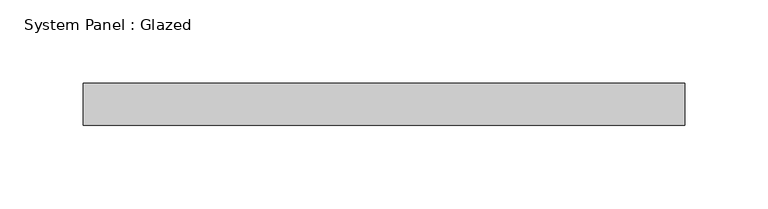
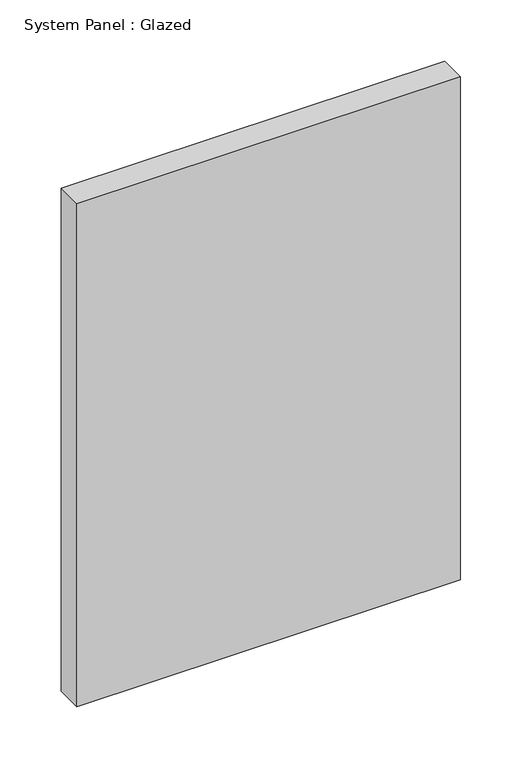
"""IFC4 building model written with IfcOpenShell, lengths in millimetres: plate geometry, System Panel : Glazed."""

from ifc_helpers import new_model, si_unit, origin, origin_with_axes, place, context, project, spatial, polyline, outline, extrude, source, transform, mapped, element, save


def system_panel_glazed_a58f4d23(model_context):
    return source(origin(), model_context, "Body", "SweptSolid", [
        extrude(outline(polyline([(180.975, 19.05), (-180.975, 19.05), (-180.975, 44.45), (180.975, 44.45), (180.975, 19.05)])), origin_with_axes(), (0.0, 0.0, 1.0), 501.65),
    ])


if __name__ == "__main__":
    model = new_model("IFC4")
    model_context = context("Model", 3, world=origin())
    ifc_project = project(units=[si_unit("LENGTHUNIT", "METRE", prefix="MILLI")], contexts=[model_context])
    site = spatial("IfcSite", under=ifc_project)
    building = spatial("IfcBuilding", under=site)
    placement = place(None, origin())
    system_panel_glazed_shape = system_panel_glazed_a58f4d23(model_context)
    element("IfcPlate", 1, ObjectType="System Panel : Glazed", at=placement, inside=building, context=model_context, shape_type="MappedRepresentation", body=[
        mapped(system_panel_glazed_shape, transform((0.0, 0.0, 0.0), x_axis=(1.0, 0.0, 0.0), y_axis=(0.0, 1.0, 0.0), z_axis=(0.0, 0.0, 1.0))),
    ])
    save(model, "model.ifc")

# Revit data of these elements
# Type "System Panel : Glazed"
#   Construction Type Id = "GSP4R"
#   Analytic Construction = "1/8 in Pilkington single glazing"
#   Visual Light Transmittance = 0.9
#   Solar Heat Gain Coefficient = 0.86
#   Heat Transfer Coefficient (U) = 1.18115 BTU/(h·ft²·°F)
#   Define Thermal Properties by = 1
# Element 1 (IfcPlate, "System Panel : Glazed")
#   Materials on its faces: "Glass"
# Materials
#   "Glass": class "Glass", colour RGB 0 128 192, transparency 0.75, Description = "Soda Lime Glass", Cost = 0
